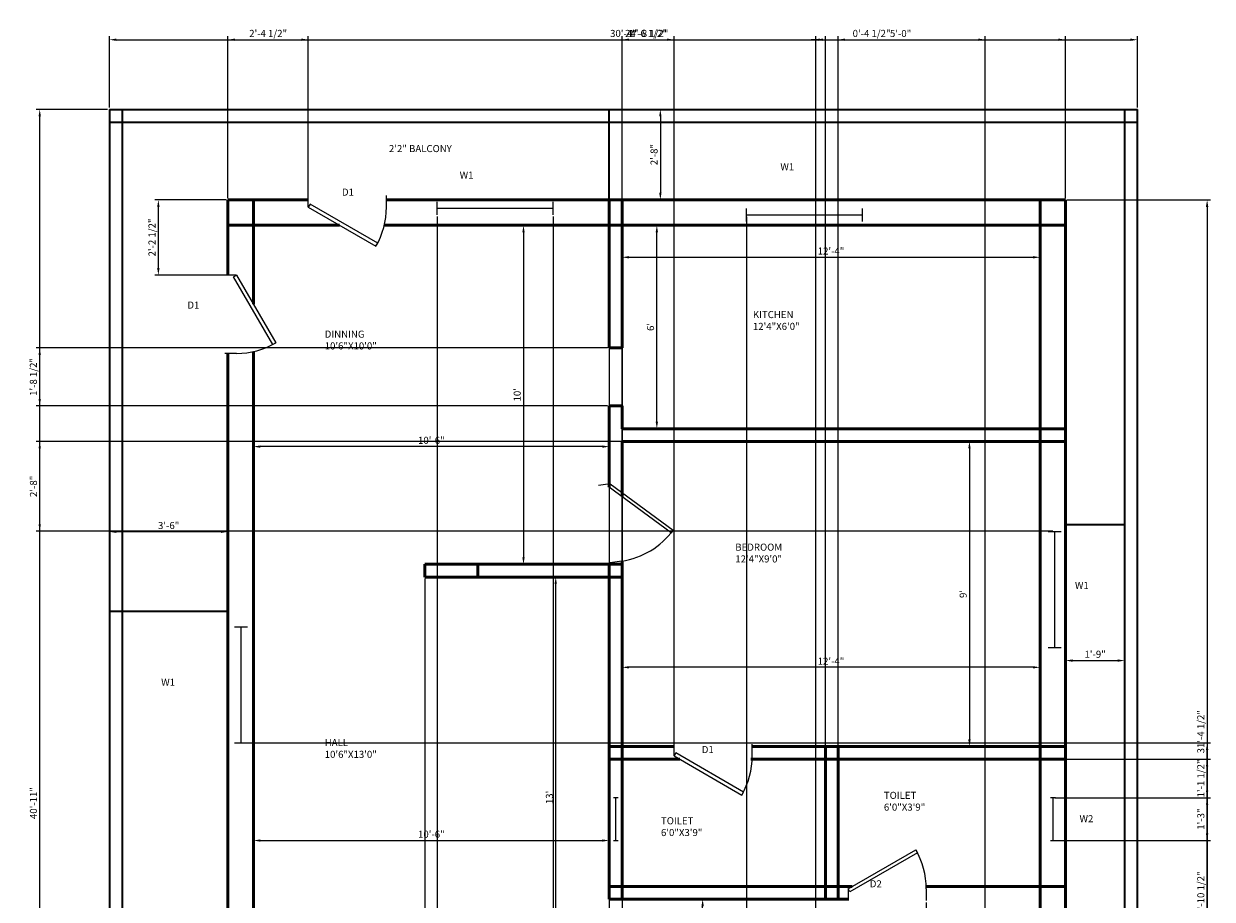
# Model space of a CAD drawing. Units: millimetres. Extents: x 2177 to 2598, y 1637 to 2185.
# Tile 2 of 2: x 2177 to 2598, y 1875 to 2185. Entities that reach past the tile are written whole.
import ezdxf

# ---------------------------------------------------------------- set-up
doc = ezdxf.new("R2010")
doc.units = ezdxf.units.MM
for name, color, linetype, lineweight in [('A-ANNO-DIMS', 150, 'Continuous', 18), ('A-ANNO-TEXT', 40, 'Continuous', 18), ('A-AREA-IDEN', 40, 'Continuous', 25), ('A-WALL-SITE', 100, 'Continuous', 35), ('door', 130, 'Continuous', 25), ('walls', 100, 'Continuous', 50), ('windows', 10, 'Continuous', 25)]:
    doc.layers.add(name, color=color, linetype=linetype, lineweight=lineweight)
doc.styles.get("Standard").update_dxf_attribs({"font": 'arial.ttf'})
doc.dimstyles.new('ISO-25', dxfattribs={"dimtxt": 2.5, "dimasz": 2.5, "dimexe": 1.25, "dimexo": 0.625, "dimtad": 1, "dimlunit": 3, "dimtxsty": 'Standard', "dimcen": 2.5, "dimadec": 0, "dimazin": 0, "dimtfac": 1, "dimtmove": 0, "dimatfit": 3, "dimfxl": 1, "dimarcsym": 0})

# ---------------------------------------------------------------- blocks, each defined once
blk = doc.blocks.new('*U2')
for p, q in [((0, 0), (0, -6)), ((40, 0), (40, -6))]:
    blk.add_line(p, q)
blk.add_lwpolyline([(0, 0), (34.64, 20), (35.52, 18.48), (0.87, -1.52)], close=True)
blk.add_arc((0, 0), 40, 0, 30)
blk = doc.blocks.new('*U4')
for p, q in [((0, 0), (0, -6)), ((40, 0), (40, -6))]:
    blk.add_line(p, q)
blk.add_lwpolyline([(0, 0), (28.28, 28.28), (29.52, 27.05), (1.24, -1.24)], close=True)
blk.add_arc((0, 0), 40, 0, 45)
blk = doc.blocks.new('*U3')
for p, q in [((0, 0), (0, 6)), ((40, 0), (40, 6))]:
    blk.add_line(p, q)
blk.add_lwpolyline([(0, 0), (34.64, -20), (35.52, -18.48), (0.87, 1.52)], close=True)
blk.add_arc((0, 0), 40, 330, 0)
blk = doc.blocks.new('*U7')
for p, q in [((0, 4), (0, 0)), ((36, 4), (36, 0)), ((0, 2), (36, 2))]:
    blk.add_line(p, q)
blk = doc.blocks.new('*D8')
at = {"layer": 'A-ANNO-DIMS', "color": 0, "lineweight": -2, "transparency": 16777216}
for p, q in [((2258.47, 2035.8), (2258.47, 2036.42)), ((2381.97, 2035.17), (2260.97, 2035.17)), ((2384.47, 2034.55), (2384.47, 2033.92))]:
    blk.add_line(p, q, dxfattribs=at)
at = {"layer": 'A-ANNO-DIMS', "color": 0, "transparency": 16777216}
for points in [[(2260.97, 2035.59), (2260.97, 2034.75), (2258.47, 2035.17)], [(2381.97, 2035.59), (2381.97, 2034.75), (2384.47, 2035.17)]]:
    blk.add_solid(points, dxfattribs=at)
at = {"layer": 'Defpoints', "color": 0, "transparency": 16777216}
for p in [(2258.47, 2035.17), (2258.47, 2035.17), (2384.47, 2035.17)]:
    blk.add_point(p, dxfattribs=at)
at = {"layer": 'A-ANNO-DIMS', "color": 0, "transparency": 16777216, "insert": (2321.47, 2037.07), "char_height": 2.5, "attachment_point": 5}
blk.add_mtext('10\'-6"', dxfattribs=at)
blk = doc.blocks.new('*D9')
at = {"layer": 'A-ANNO-DIMS', "color": 0, "lineweight": -2, "transparency": 16777216}
for p, q in [((2338.03, 2113.52), (2355.34, 2113.52)), ((2354.09, 2111.02), (2354.09, 1996.02)), ((2338.03, 1993.52), (2355.34, 1993.52))]:
    blk.add_line(p, q, dxfattribs=at)
at = {"layer": 'A-ANNO-DIMS', "color": 0, "transparency": 16777216}
for points in [[(2353.68, 2111.02), (2354.51, 2111.02), (2354.09, 2113.52)], [(2353.68, 1996.02), (2354.51, 1996.02), (2354.09, 1993.52)]]:
    blk.add_solid(points, dxfattribs=at)
at = {"layer": 'Defpoints', "color": 0, "transparency": 16777216}
for p in [(2337.4, 2113.52), (2337.4, 1993.52), (2354.09, 1993.52)]:
    blk.add_point(p, dxfattribs=at)
at = {"layer": 'A-ANNO-DIMS', "color": 0, "transparency": 16777216, "insert": (2352.19, 2053.52), "char_height": 2.5, "attachment_point": 5, "rotation": 90}
blk.add_mtext("10'", dxfattribs=at)
blk = doc.blocks.new('*D10')
at = {"layer": 'A-ANNO-DIMS', "color": 0, "lineweight": -2, "transparency": 16777216}
for p, q in [((2417.03, 2113.52), (2400.05, 2113.52)), ((2401.3, 2044.02), (2401.3, 2111.02)), ((2417.03, 2041.52), (2400.05, 2041.52))]:
    blk.add_line(p, q, dxfattribs=at)
at = {"layer": 'A-ANNO-DIMS', "color": 0, "transparency": 16777216}
for points in [[(2400.89, 2111.02), (2401.72, 2111.02), (2401.3, 2113.52)], [(2400.89, 2044.02), (2401.72, 2044.02), (2401.3, 2041.52)]]:
    blk.add_solid(points, dxfattribs=at)
at = {"layer": 'Defpoints', "color": 0, "transparency": 16777216}
for p in [(2401.3, 2113.52), (2417.66, 2113.52), (2417.66, 2041.52)]:
    blk.add_point(p, dxfattribs=at)
at = {"layer": 'A-ANNO-DIMS', "color": 0, "transparency": 16777216, "insert": (2399.4, 2077.52), "char_height": 2.5, "attachment_point": 5, "rotation": 90}
blk.add_mtext("6'", dxfattribs=at)
blk = doc.blocks.new('*D11')
at = {"layer": 'A-ANNO-DIMS', "color": 0, "lineweight": -2, "transparency": 16777216}
for p, q in [((2388.97, 2087.6), (2388.97, 2103.44)), ((2391.47, 2102.19), (2534.47, 2102.19)), ((2536.97, 2087.6), (2536.97, 2103.44))]:
    blk.add_line(p, q, dxfattribs=at)
at = {"layer": 'A-ANNO-DIMS', "color": 0, "transparency": 16777216}
for points in [[(2391.47, 2102.6), (2391.47, 2101.77), (2388.97, 2102.19)], [(2534.47, 2102.6), (2534.47, 2101.77), (2536.97, 2102.19)]]:
    blk.add_solid(points, dxfattribs=at)
at = {"layer": 'Defpoints', "color": 0, "transparency": 16777216}
for p in [(2536.97, 2102.19), (2388.97, 2086.97), (2536.97, 2086.97)]:
    blk.add_point(p, dxfattribs=at)
at = {"layer": 'A-ANNO-DIMS', "color": 0, "transparency": 16777216, "insert": (2462.97, 2104.07), "char_height": 2.5, "attachment_point": 5}
blk.add_mtext('12\'-4"', dxfattribs=at)
blk = doc.blocks.new('*D12')
at = {"layer": 'A-ANNO-DIMS', "color": 0, "lineweight": -2, "transparency": 16777216}
for p, q in [((2388.97, 1957.69), (2388.97, 1958.31)), ((2534.47, 1957.06), (2391.47, 1957.06)), ((2536.97, 1957.69), (2536.97, 1958.31))]:
    blk.add_line(p, q, dxfattribs=at)
at = {"layer": 'A-ANNO-DIMS', "color": 0, "transparency": 16777216}
for points in [[(2391.47, 1957.48), (2391.47, 1956.65), (2388.97, 1957.06)], [(2534.47, 1957.48), (2534.47, 1956.65), (2536.97, 1957.06)]]:
    blk.add_solid(points, dxfattribs=at)
at = {"layer": 'Defpoints', "color": 0, "transparency": 16777216}
for p in [(2388.97, 1957.06), (2388.97, 1957.06), (2536.97, 1957.06)]:
    blk.add_point(p, dxfattribs=at)
at = {"layer": 'A-ANNO-DIMS', "color": 0, "transparency": 16777216, "insert": (2462.97, 1958.94), "char_height": 2.5, "attachment_point": 5}
blk.add_mtext('12\'-4"', dxfattribs=at)
blk = doc.blocks.new('*D13')
at = {"layer": 'A-ANNO-DIMS', "color": 0, "lineweight": -2, "transparency": 16777216}
for p, q in [((2468.09, 2037.02), (2513.23, 2037.02)), ((2511.98, 2034.52), (2511.98, 1931.52)), ((2468.09, 1929.02), (2513.23, 1929.02))]:
    blk.add_line(p, q, dxfattribs=at)
at = {"layer": 'A-ANNO-DIMS', "color": 0, "transparency": 16777216}
for points in [[(2511.56, 2034.52), (2512.4, 2034.52), (2511.98, 2037.02)], [(2511.56, 1931.52), (2512.4, 1931.52), (2511.98, 1929.02)]]:
    blk.add_solid(points, dxfattribs=at)
at = {"layer": 'Defpoints', "color": 0, "transparency": 16777216}
for p in [(2467.47, 2037.02), (2467.47, 1929.02), (2511.98, 1929.02)]:
    blk.add_point(p, dxfattribs=at)
at = {"layer": 'A-ANNO-DIMS', "color": 0, "transparency": 16777216, "insert": (2510.08, 1983.02), "char_height": 2.5, "attachment_point": 5, "rotation": 90}
blk.add_mtext("9'", dxfattribs=at)
blk = doc.blocks.new('*D14')
at = {"layer": 'A-ANNO-DIMS', "color": 0, "lineweight": -2, "transparency": 16777216}
for p, q in [((2258.47, 1888.11), (2258.47, 1897.01)), ((2260.97, 1895.76), (2381.97, 1895.76)), ((2384.47, 1888.11), (2384.47, 1897.01))]:
    blk.add_line(p, q, dxfattribs=at)
at = {"layer": 'A-ANNO-DIMS', "color": 0, "transparency": 16777216}
for points in [[(2260.97, 1896.18), (2260.97, 1895.35), (2258.47, 1895.76)], [(2381.97, 1896.18), (2381.97, 1895.35), (2384.47, 1895.76)]]:
    blk.add_solid(points, dxfattribs=at)
at = {"layer": 'Defpoints', "color": 0, "transparency": 16777216}
for p in [(2384.47, 1895.76), (2258.47, 1887.49), (2384.47, 1887.49)]:
    blk.add_point(p, dxfattribs=at)
at = {"layer": 'A-ANNO-DIMS', "color": 0, "transparency": 16777216, "insert": (2321.47, 1897.67), "char_height": 2.5, "attachment_point": 5}
blk.add_mtext('10\'-6"', dxfattribs=at)
blk = doc.blocks.new('*D15')
at = {"layer": 'A-ANNO-DIMS', "color": 0, "lineweight": -2, "transparency": 16777216}
for p, q in [((2344.56, 1989.02), (2366.75, 1989.02)), ((2365.5, 1835.52), (2365.5, 1986.52)), ((2344.56, 1833.02), (2366.75, 1833.02))]:
    blk.add_line(p, q, dxfattribs=at)
at = {"layer": 'A-ANNO-DIMS', "color": 0, "transparency": 16777216}
for points in [[(2365.08, 1986.52), (2365.91, 1986.52), (2365.5, 1989.02)], [(2365.08, 1835.52), (2365.91, 1835.52), (2365.5, 1833.02)]]:
    blk.add_solid(points, dxfattribs=at)
at = {"layer": 'Defpoints', "color": 0, "transparency": 16777216}
for p in [(2343.93, 1989.02), (2365.5, 1989.02), (2343.93, 1833.02)]:
    blk.add_point(p, dxfattribs=at)
at = {"layer": 'A-ANNO-DIMS', "color": 0, "transparency": 16777216, "insert": (2363.59, 1911.02), "char_height": 2.5, "attachment_point": 5, "rotation": 90}
blk.add_mtext("13'", dxfattribs=at)
blk = doc.blocks.new('*D18')
at = {"layer": 'A-ANNO-DIMS', "color": 0, "lineweight": -2, "transparency": 16777216}
for p, q in [((2417.52, 1757.52), (2417.52, 1872.52)), ((2418.14, 1875.02), (2418.77, 1875.02)), ((2418.14, 1755.02), (2418.77, 1755.02))]:
    blk.add_line(p, q, dxfattribs=at)
at = {"layer": 'A-ANNO-DIMS', "color": 0, "transparency": 16777216}
for points in [[(2417.1, 1872.52), (2417.93, 1872.52), (2417.52, 1875.02)], [(2417.1, 1757.52), (2417.93, 1757.52), (2417.52, 1755.02)]]:
    blk.add_solid(points, dxfattribs=at)
at = {"layer": 'Defpoints', "color": 0, "transparency": 16777216}
for p in [(2417.52, 1875.02), (2417.52, 1875.02), (2417.52, 1755.02)]:
    blk.add_point(p, dxfattribs=at)
at = {"layer": 'A-ANNO-DIMS', "color": 0, "transparency": 16777216, "insert": (2415.61, 1815.02), "char_height": 2.5, "attachment_point": 5, "rotation": 90}
blk.add_mtext("10'", dxfattribs=at)
blk = doc.blocks.new('*D20')
at = {"layer": 'A-ANNO-DIMS', "color": 0, "lineweight": -2, "transparency": 16777216}
for p, q in [((2545.97, 1934.9), (2545.97, 1960.7)), ((2548.47, 1959.45), (2564.47, 1959.45)), ((2566.97, 1934.9), (2566.97, 1960.7))]:
    blk.add_line(p, q, dxfattribs=at)
at = {"layer": 'A-ANNO-DIMS', "color": 0, "transparency": 16777216}
for points in [[(2548.47, 1959.87), (2548.47, 1959.03), (2545.97, 1959.45)], [(2564.47, 1959.87), (2564.47, 1959.03), (2566.97, 1959.45)]]:
    blk.add_solid(points, dxfattribs=at)
at = {"layer": 'Defpoints', "color": 0, "transparency": 16777216}
for p in [(2566.97, 1959.45), (2545.97, 1934.27), (2566.97, 1934.27)]:
    blk.add_point(p, dxfattribs=at)
at = {"layer": 'A-ANNO-DIMS', "color": 0, "transparency": 16777216, "insert": (2556.47, 1961.35), "char_height": 2.5, "attachment_point": 5}
blk.add_mtext('1\'-9"', dxfattribs=at)
blk = doc.blocks.new('*D21')
at = {"layer": 'A-ANNO-DIMS', "color": 0, "lineweight": -2, "transparency": 16777216}
for p, q in [((2398.56, 2154.52), (2403.79, 2154.52)), ((2402.54, 2152.02), (2402.54, 2125.02)), ((2398.56, 2122.52), (2403.79, 2122.52))]:
    blk.add_line(p, q, dxfattribs=at)
at = {"layer": 'A-ANNO-DIMS', "color": 0, "transparency": 16777216}
for points in [[(2402.13, 2152.02), (2402.96, 2152.02), (2402.54, 2154.52)], [(2402.13, 2125.02), (2402.96, 2125.02), (2402.54, 2122.52)]]:
    blk.add_solid(points, dxfattribs=at)
at = {"layer": 'Defpoints', "color": 0, "transparency": 16777216}
for p in [(2397.93, 2154.52), (2397.93, 2122.52), (2402.54, 2122.52)]:
    blk.add_point(p, dxfattribs=at)
at = {"layer": 'A-ANNO-DIMS', "color": 0, "transparency": 16777216, "insert": (2400.64, 2138.52), "char_height": 2.5, "attachment_point": 5, "rotation": 90}
blk.add_mtext('2\'-8"', dxfattribs=at)
blk = doc.blocks.new('*D22')
at = {"layer": 'A-ANNO-DIMS', "color": 0, "lineweight": -2, "transparency": 16777216}
for p, q in [((2207.47, 1992.8), (2207.47, 2006.28)), ((2246.97, 2005.03), (2209.97, 2005.03)), ((2249.47, 1992.8), (2249.47, 2006.28))]:
    blk.add_line(p, q, dxfattribs=at)
at = {"layer": 'A-ANNO-DIMS', "color": 0, "transparency": 16777216}
for points in [[(2209.97, 2005.44), (2209.97, 2004.61), (2207.47, 2005.03)], [(2246.97, 2005.44), (2246.97, 2004.61), (2249.47, 2005.03)]]:
    blk.add_solid(points, dxfattribs=at)
at = {"layer": 'Defpoints', "color": 0, "transparency": 16777216}
for p in [(2207.47, 2005.03), (2207.47, 1992.17), (2249.47, 1992.17)]:
    blk.add_point(p, dxfattribs=at)
at = {"layer": 'A-ANNO-DIMS', "color": 0, "transparency": 16777216, "insert": (2228.47, 2006.93), "char_height": 2.5, "attachment_point": 5}
blk.add_mtext('3\'-6"', dxfattribs=at)
blk = doc.blocks.new('*D23')
at = {"layer": 'A-ANNO-DIMS', "color": 0, "lineweight": -2, "transparency": 16777216}
for p, q in [((2248.84, 2122.52), (2223.57, 2122.52)), ((2224.82, 2098.33), (2224.82, 2120.02)), ((2248.84, 2095.83), (2223.57, 2095.83))]:
    blk.add_line(p, q, dxfattribs=at)
at = {"layer": 'A-ANNO-DIMS', "color": 0, "transparency": 16777216}
for points in [[(2224.4, 2120.02), (2225.24, 2120.02), (2224.82, 2122.52)], [(2224.4, 2098.33), (2225.24, 2098.33), (2224.82, 2095.83)]]:
    blk.add_solid(points, dxfattribs=at)
at = {"layer": 'Defpoints', "color": 0, "transparency": 16777216}
for p in [(2224.82, 2122.52), (2249.47, 2122.52), (2249.47, 2095.83)]:
    blk.add_point(p, dxfattribs=at)
at = {"layer": 'A-ANNO-DIMS', "color": 0, "transparency": 16777216, "insert": (2222.9, 2109.18), "char_height": 2.5, "attachment_point": 5, "rotation": 90}
blk.add_mtext('2\'-2 1/2"', dxfattribs=at)
blk = doc.blocks.new('*D24')
at = {"layer": 'A-ANNO-DIMS', "color": 0, "lineweight": -2, "transparency": 16777216}
for p, q in [((2207.47, 2155.15), (2207.47, 2180.42)), ((2571.47, 2155.15), (2571.47, 2180.42)), ((2209.97, 2179.17), (2568.97, 2179.17))]:
    blk.add_line(p, q, dxfattribs=at)
at = {"layer": 'A-ANNO-DIMS', "color": 0, "transparency": 16777216}
for points in [[(2209.97, 2179.59), (2209.97, 2178.76), (2207.47, 2179.17)], [(2568.97, 2179.59), (2568.97, 2178.76), (2571.47, 2179.17)]]:
    blk.add_solid(points, dxfattribs=at)
at = {"layer": 'Defpoints', "color": 0, "transparency": 16777216}
for p in [(2571.47, 2179.17), (2207.47, 2154.52), (2571.47, 2154.52)]:
    blk.add_point(p, dxfattribs=at)
at = {"layer": 'A-ANNO-DIMS', "color": 0, "transparency": 16777216, "insert": (2389.47, 2181.08), "char_height": 2.5, "attachment_point": 5}
blk.add_mtext('30\'-4"', dxfattribs=at)
blk = doc.blocks.new('*D25')
at = {"layer": 'A-ANNO-DIMS', "color": 0, "lineweight": -2, "transparency": 16777216}
for p, q in [((2206.84, 2154.52), (2181.57, 2154.52)), ((2182.82, 1666.02), (2182.82, 2152.02)), ((2206.84, 1663.52), (2181.57, 1663.52))]:
    blk.add_line(p, q, dxfattribs=at)
at = {"layer": 'A-ANNO-DIMS', "color": 0, "transparency": 16777216}
for points in [[(2182.4, 2152.02), (2183.24, 2152.02), (2182.82, 2154.52)], [(2182.4, 1666.02), (2183.24, 1666.02), (2182.82, 1663.52)]]:
    blk.add_solid(points, dxfattribs=at)
at = {"layer": 'Defpoints', "color": 0, "transparency": 16777216}
for p in [(2182.82, 2154.52), (2207.47, 2154.52), (2207.47, 1663.52)]:
    blk.add_point(p, dxfattribs=at)
at = {"layer": 'A-ANNO-DIMS', "color": 0, "transparency": 16777216, "insert": (2180.92, 1909.02), "char_height": 2.5, "attachment_point": 5, "rotation": 90}
blk.add_mtext('40\'-11"', dxfattribs=at)
blk = doc.blocks.new('*D26')
at = {"layer": 'A-ANNO-DIMS', "color": 0, "lineweight": -2, "transparency": 16777216}
for p, q in [((2249.47, 2123.15), (2249.47, 2180.42)), ((2545.97, 2123.15), (2545.97, 2180.42)), ((2251.97, 2179.17), (2543.47, 2179.17))]:
    blk.add_line(p, q, dxfattribs=at)
at = {"layer": 'A-ANNO-DIMS', "color": 0, "transparency": 16777216}
for points in [[(2251.97, 2179.59), (2251.97, 2178.76), (2249.47, 2179.17)], [(2543.47, 2179.59), (2543.47, 2178.76), (2545.97, 2179.17)]]:
    blk.add_solid(points, dxfattribs=at)
at = {"layer": 'Defpoints', "color": 0, "transparency": 16777216}
for p in [(2545.97, 2179.17), (2249.47, 2122.52), (2545.97, 2122.52)]:
    blk.add_point(p, dxfattribs=at)
at = {"layer": 'A-ANNO-DIMS', "color": 0, "transparency": 16777216, "insert": (2397.72, 2181.09), "char_height": 2.5, "attachment_point": 5}
blk.add_mtext('24\'-8 1/2"', dxfattribs=at)
blk = doc.blocks.new('*D27')
at = {"layer": 'A-ANNO-DIMS', "color": 0, "lineweight": -2, "transparency": 16777216}
for p, q in [((2546.59, 2122.52), (2597.37, 2122.52)), ((2596.12, 2120.02), (2596.12, 1748.52)), ((2546.59, 1746.02), (2597.37, 1746.02))]:
    blk.add_line(p, q, dxfattribs=at)
at = {"layer": 'A-ANNO-DIMS', "color": 0, "transparency": 16777216}
for points in [[(2595.7, 2120.02), (2596.54, 2120.02), (2596.12, 2122.52)], [(2595.7, 1748.52), (2596.54, 1748.52), (2596.12, 1746.02)]]:
    blk.add_solid(points, dxfattribs=at)
at = {"layer": 'Defpoints', "color": 0, "transparency": 16777216}
for p in [(2545.97, 2122.52), (2545.97, 1746.02), (2596.12, 1746.02)]:
    blk.add_point(p, dxfattribs=at)
at = {"layer": 'A-ANNO-DIMS', "color": 0, "transparency": 16777216, "insert": (2594.2, 1934.27), "char_height": 2.5, "attachment_point": 5, "rotation": 90}
blk.add_mtext('31\'-4 1/2"', dxfattribs=at)
blk = doc.blocks.new('*D29')
at = {"layer": 'A-ANNO-DIMS', "color": 0, "lineweight": -2, "transparency": 16777216}
for p, q in [((2460.97, 1929.65), (2460.97, 2180.42)), ((2465.47, 1929.65), (2465.47, 2180.42)), ((2458.47, 2179.17), (2455.97, 2179.17)), ((2460.97, 2179.17), (2465.47, 2179.17)), ((2467.97, 2179.17), (2484.19, 2179.17))]:
    blk.add_line(p, q, dxfattribs=at)
at = {"layer": 'A-ANNO-DIMS', "color": 0, "transparency": 16777216}
for points in [[(2458.47, 2179.59), (2458.47, 2178.76), (2460.97, 2179.17)], [(2467.97, 2179.59), (2467.97, 2178.76), (2465.47, 2179.17)]]:
    blk.add_solid(points, dxfattribs=at)
at = {"layer": 'Defpoints', "color": 0, "transparency": 16777216}
for p in [(2465.47, 2179.17), (2460.97, 1929.02), (2465.47, 1929.02)]:
    blk.add_point(p, dxfattribs=at)
at = {"layer": 'A-ANNO-DIMS', "color": 0, "transparency": 16777216, "insert": (2477.33, 2181.09), "char_height": 2.5, "attachment_point": 5}
blk.add_mtext('0\'-4 1/2"', dxfattribs=at)
blk = doc.blocks.new('*D33')
at = {"layer": 'A-ANNO-DIMS', "color": 0, "lineweight": -2, "transparency": 16777216}
for p, q in [((2323.55, 2116.57), (2323.55, 1637.62)), ((2364.65, 2116.57), (2364.65, 1637.62)), ((2326.05, 1638.87), (2362.15, 1638.87))]:
    blk.add_line(p, q, dxfattribs=at)
at = {"layer": 'A-ANNO-DIMS', "color": 0, "transparency": 16777216}
for points in [[(2326.05, 1639.29), (2326.05, 1638.46), (2323.55, 1638.87)], [(2362.15, 1639.29), (2362.15, 1638.46), (2364.65, 1638.87)]]:
    blk.add_solid(points, dxfattribs=at)
at = {"layer": 'Defpoints', "color": 0, "transparency": 16777216}
for p in [(2323.55, 2117.19), (2364.65, 2117.19), (2364.65, 1638.87)]:
    blk.add_point(p, dxfattribs=at)
at = {"layer": 'A-ANNO-DIMS', "color": 0, "transparency": 16777216, "insert": (2344.1, 1640.78), "char_height": 2.5, "attachment_point": 5}
blk.add_mtext('3\'-5"', dxfattribs=at)
blk = doc.blocks.new('*D34')
at = {"layer": 'A-ANNO-DIMS', "color": 0, "lineweight": -2, "transparency": 16777216}
for p, q in [((2542.2, 1910.93), (2597.37, 1910.93)), ((2596.12, 1908.43), (2596.12, 1898.25)), ((2542.2, 1895.75), (2597.37, 1895.75))]:
    blk.add_line(p, q, dxfattribs=at)
at = {"layer": 'A-ANNO-DIMS', "color": 0, "transparency": 16777216}
for points in [[(2595.7, 1908.43), (2596.54, 1908.43), (2596.12, 1910.93)], [(2595.7, 1898.25), (2596.54, 1898.25), (2596.12, 1895.75)]]:
    blk.add_solid(points, dxfattribs=at)
at = {"layer": 'Defpoints', "color": 0, "transparency": 16777216}
for p in [(2541.57, 1910.93), (2541.57, 1895.75), (2596.12, 1895.75)]:
    blk.add_point(p, dxfattribs=at)
at = {"layer": 'A-ANNO-DIMS', "color": 0, "transparency": 16777216, "insert": (2594.22, 1903.34), "char_height": 2.5, "attachment_point": 5, "rotation": 90}
blk.add_mtext('1\'-3"', dxfattribs=at)
blk = doc.blocks.new('*D35')
at = {"layer": 'A-ANNO-DIMS', "color": 0, "lineweight": -2, "transparency": 16777216}
for p, q in [((2457.6, 1746.65), (2457.6, 2180.42)), ((2517.6, 1746.65), (2517.6, 2180.42)), ((2460.1, 2179.17), (2515.1, 2179.17))]:
    blk.add_line(p, q, dxfattribs=at)
at = {"layer": 'A-ANNO-DIMS', "color": 0, "transparency": 16777216}
for points in [[(2460.1, 2179.59), (2460.1, 2178.76), (2457.6, 2179.17)], [(2515.1, 2179.59), (2515.1, 2178.76), (2517.6, 2179.17)]]:
    blk.add_solid(points, dxfattribs=at)
at = {"layer": 'Defpoints', "color": 0, "transparency": 16777216}
for p in [(2517.6, 2179.17), (2457.6, 1746.02), (2517.6, 1746.02)]:
    blk.add_point(p, dxfattribs=at)
at = {"layer": 'A-ANNO-DIMS', "color": 0, "transparency": 16777216, "insert": (2487.6, 2181.07), "char_height": 2.5, "attachment_point": 5}
blk.add_mtext('5\'-0"', dxfattribs=at)
blk = doc.blocks.new('*D42')
at = {"layer": 'A-ANNO-DIMS', "color": 0, "lineweight": -2, "transparency": 16777216}
for p, q in [((2388.97, 1929.65), (2388.97, 2180.42)), ((2407.39, 1929.65), (2407.39, 2180.42)), ((2391.47, 2179.17), (2404.89, 2179.17))]:
    blk.add_line(p, q, dxfattribs=at)
at = {"layer": 'A-ANNO-DIMS', "color": 0, "transparency": 16777216}
for points in [[(2391.47, 2179.59), (2391.47, 2178.76), (2388.97, 2179.17)], [(2404.89, 2179.59), (2404.89, 2178.76), (2407.39, 2179.17)]]:
    blk.add_solid(points, dxfattribs=at)
at = {"layer": 'Defpoints', "color": 0, "transparency": 16777216}
for p in [(2407.39, 2179.17), (2388.97, 1929.02), (2407.39, 1929.02)]:
    blk.add_point(p, dxfattribs=at)
at = {"layer": 'A-ANNO-DIMS', "color": 0, "transparency": 16777216, "insert": (2398.18, 2181.09), "char_height": 2.5, "attachment_point": 5}
blk.add_mtext('1\'-6 1/2"', dxfattribs=at)
blk = doc.blocks.new('*D43')
at = {"layer": 'A-ANNO-DIMS', "color": 0, "lineweight": -2, "transparency": 16777216}
for p, q in [((2545.97, 1878.9), (2545.97, 1637.62)), ((2496.67, 1873.88), (2496.67, 1637.62)), ((2499.17, 1638.87), (2543.47, 1638.87))]:
    blk.add_line(p, q, dxfattribs=at)
at = {"layer": 'A-ANNO-DIMS', "color": 0, "transparency": 16777216}
for points in [[(2499.17, 1639.29), (2499.17, 1638.46), (2496.67, 1638.87)], [(2543.47, 1639.29), (2543.47, 1638.46), (2545.97, 1638.87)]]:
    blk.add_solid(points, dxfattribs=at)
at = {"layer": 'Defpoints', "color": 0, "transparency": 16777216}
for p in [(2545.97, 1879.52), (2496.67, 1874.51), (2545.97, 1638.87)]:
    blk.add_point(p, dxfattribs=at)
at = {"layer": 'A-ANNO-DIMS', "color": 0, "transparency": 16777216, "insert": (2521.32, 1640.79), "char_height": 2.5, "attachment_point": 5}
blk.add_mtext('4\'-1 1/2"', dxfattribs=at)
blk = doc.blocks.new('*D44')
at = {"layer": 'A-ANNO-DIMS', "color": 0, "lineweight": -2, "transparency": 16777216}
for p, q in [((2546.59, 1924.52), (2597.37, 1924.52)), ((2596.12, 1913.43), (2596.12, 1922.02)), ((2542.2, 1910.93), (2597.37, 1910.93))]:
    blk.add_line(p, q, dxfattribs=at)
at = {"layer": 'A-ANNO-DIMS', "color": 0, "transparency": 16777216}
for points in [[(2595.7, 1922.02), (2596.54, 1922.02), (2596.12, 1924.52)], [(2595.7, 1913.43), (2596.54, 1913.43), (2596.12, 1910.93)]]:
    blk.add_solid(points, dxfattribs=at)
at = {"layer": 'Defpoints', "color": 0, "transparency": 16777216}
for p in [(2545.97, 1924.52), (2596.12, 1924.52), (2541.57, 1910.93)]:
    blk.add_point(p, dxfattribs=at)
at = {"layer": 'A-ANNO-DIMS', "color": 0, "transparency": 16777216, "insert": (2594.2, 1917.73), "char_height": 2.5, "attachment_point": 5, "rotation": 90}
blk.add_mtext('1\'-1 1/2"', dxfattribs=at)
blk = doc.blocks.new('*D46')
at = {"layer": 'A-ANNO-DIMS', "color": 0, "lineweight": -2, "transparency": 16777216}
for p, q in [((2383.84, 2070.11), (2181.57, 2070.11)), ((2182.82, 2052.05), (2182.82, 2067.61)), ((2383.84, 2049.55), (2181.57, 2049.55))]:
    blk.add_line(p, q, dxfattribs=at)
at = {"layer": 'A-ANNO-DIMS', "color": 0, "transparency": 16777216}
for points in [[(2182.4, 2067.61), (2183.24, 2067.61), (2182.82, 2070.11)], [(2182.4, 2052.05), (2183.24, 2052.05), (2182.82, 2049.55)]]:
    blk.add_solid(points, dxfattribs=at)
at = {"layer": 'Defpoints', "color": 0, "transparency": 16777216}
for p in [(2182.82, 2070.11), (2384.47, 2070.11), (2384.47, 2049.55)]:
    blk.add_point(p, dxfattribs=at)
at = {"layer": 'A-ANNO-DIMS', "color": 0, "transparency": 16777216, "insert": (2180.9, 2059.83), "char_height": 2.5, "attachment_point": 5, "rotation": 90}
blk.add_mtext('1\'-8 1/2"', dxfattribs=at)
blk = doc.blocks.new('*D47')
at = {"layer": 'A-ANNO-DIMS', "color": 0, "lineweight": -2, "transparency": 16777216}
for p, q in [((2319.22, 1988.4), (2319.22, 1637.62)), ((2388.97, 1988.4), (2388.97, 1637.62)), ((2321.72, 1638.87), (2386.47, 1638.87))]:
    blk.add_line(p, q, dxfattribs=at)
at = {"layer": 'A-ANNO-DIMS', "color": 0, "transparency": 16777216}
for points in [[(2321.72, 1639.29), (2321.72, 1638.46), (2319.22, 1638.87)], [(2386.47, 1639.29), (2386.47, 1638.46), (2388.97, 1638.87)]]:
    blk.add_solid(points, dxfattribs=at)
at = {"layer": 'Defpoints', "color": 0, "transparency": 16777216}
for p in [(2319.22, 1989.02), (2388.97, 1989.02), (2388.97, 1638.87)]:
    blk.add_point(p, dxfattribs=at)
at = {"layer": 'A-ANNO-DIMS', "color": 0, "transparency": 16777216, "insert": (2354.09, 1640.77), "char_height": 2.5, "attachment_point": 5}
blk.add_mtext('5\'-10"', dxfattribs=at)
blk = doc.blocks.new('*D48')
at = {"layer": 'A-ANNO-DIMS', "color": 0, "lineweight": -2, "transparency": 16777216}
for p, q in [((2388.97, 2121.9), (2388.97, 1637.62)), ((2433.07, 2116.49), (2433.07, 1637.62)), ((2391.47, 1638.87), (2430.57, 1638.87))]:
    blk.add_line(p, q, dxfattribs=at)
at = {"layer": 'A-ANNO-DIMS', "color": 0, "transparency": 16777216}
for points in [[(2391.47, 1639.29), (2391.47, 1638.46), (2388.97, 1638.87)], [(2430.57, 1639.29), (2430.57, 1638.46), (2433.07, 1638.87)]]:
    blk.add_solid(points, dxfattribs=at)
at = {"layer": 'Defpoints', "color": 0, "transparency": 16777216}
for p in [(2388.97, 2122.52), (2433.07, 2117.11), (2433.07, 1638.87)]:
    blk.add_point(p, dxfattribs=at)
at = {"layer": 'A-ANNO-DIMS', "color": 0, "transparency": 16777216, "insert": (2411.02, 1640.78), "char_height": 2.5, "attachment_point": 5}
blk.add_mtext('3\'-8"', dxfattribs=at)
blk = doc.blocks.new('*D49')
at = {"layer": 'A-ANNO-DIMS', "color": 0, "lineweight": -2, "transparency": 16777216}
for p, q in [((2249.47, 2123.15), (2249.47, 2180.42)), ((2277.91, 2123.15), (2277.91, 2180.42)), ((2251.97, 2179.17), (2275.41, 2179.17))]:
    blk.add_line(p, q, dxfattribs=at)
at = {"layer": 'A-ANNO-DIMS', "color": 0, "transparency": 16777216}
for points in [[(2251.97, 2179.59), (2251.97, 2178.76), (2249.47, 2179.17)], [(2275.41, 2179.59), (2275.41, 2178.76), (2277.91, 2179.17)]]:
    blk.add_solid(points, dxfattribs=at)
at = {"layer": 'Defpoints', "color": 0, "transparency": 16777216}
for p in [(2277.91, 2179.17), (2249.47, 2122.52), (2277.91, 2122.52)]:
    blk.add_point(p, dxfattribs=at)
at = {"layer": 'A-ANNO-DIMS', "color": 0, "transparency": 16777216, "insert": (2263.69, 2181.09), "char_height": 2.5, "attachment_point": 5}
blk.add_mtext('2\'-4 1/2"', dxfattribs=at)
blk = doc.blocks.new('*D50')
at = {"layer": 'A-ANNO-DIMS', "color": 0, "lineweight": -2, "transparency": 16777216}
for p, q in [((2254.73, 1930.31), (2597.37, 1930.31)), ((2596.12, 1826.52), (2596.12, 1927.81)), ((2259.09, 1824.02), (2597.37, 1824.02))]:
    blk.add_line(p, q, dxfattribs=at)
at = {"layer": 'A-ANNO-DIMS', "color": 0, "transparency": 16777216}
for points in [[(2595.7, 1927.81), (2596.54, 1927.81), (2596.12, 1930.31)], [(2595.7, 1826.52), (2596.54, 1826.52), (2596.12, 1824.02)]]:
    blk.add_solid(points, dxfattribs=at)
at = {"layer": 'Defpoints', "color": 0, "transparency": 16777216}
for p in [(2254.11, 1930.31), (2596.12, 1930.31), (2258.47, 1824.02)]:
    blk.add_point(p, dxfattribs=at)
at = {"layer": 'A-ANNO-DIMS', "color": 0, "transparency": 16777216, "insert": (2594.2, 1877.17), "char_height": 2.5, "attachment_point": 5, "rotation": 90}
blk.add_mtext('8\'-10 1/2"', dxfattribs=at)
blk = doc.blocks.new('*D51')
at = {"layer": 'A-ANNO-DIMS', "color": 0, "lineweight": -2, "transparency": 16777216}
for p, q in [((2545.34, 2037.02), (2181.57, 2037.02)), ((2182.82, 2007.69), (2182.82, 2034.52)), ((2541.54, 2005.19), (2181.57, 2005.19))]:
    blk.add_line(p, q, dxfattribs=at)
at = {"layer": 'A-ANNO-DIMS', "color": 0, "transparency": 16777216}
for points in [[(2182.4, 2034.52), (2183.24, 2034.52), (2182.82, 2037.02)], [(2182.4, 2007.69), (2183.24, 2007.69), (2182.82, 2005.19)]]:
    blk.add_solid(points, dxfattribs=at)
at = {"layer": 'Defpoints', "color": 0, "transparency": 16777216}
for p in [(2182.82, 2037.02), (2545.97, 2037.02), (2542.17, 2005.19)]:
    blk.add_point(p, dxfattribs=at)
at = {"layer": 'A-ANNO-DIMS', "color": 0, "transparency": 16777216, "insert": (2180.92, 2021.11), "char_height": 2.5, "attachment_point": 5, "rotation": 90}
blk.add_mtext('2\'-8"', dxfattribs=at)
blk = doc.blocks.new('*D53')
at = {"layer": 'A-ANNO-DIMS', "color": 0, "lineweight": -2, "transparency": 16777216}
for p, q in [((2384.47, 2121.9), (2384.47, 1637.62)), ((2364.65, 2116.57), (2364.65, 1637.62)), ((2367.15, 1638.87), (2381.97, 1638.87))]:
    blk.add_line(p, q, dxfattribs=at)
at = {"layer": 'A-ANNO-DIMS', "color": 0, "transparency": 16777216}
for points in [[(2367.15, 1639.29), (2367.15, 1638.46), (2364.65, 1638.87)], [(2381.97, 1639.29), (2381.97, 1638.46), (2384.47, 1638.87)]]:
    blk.add_solid(points, dxfattribs=at)
at = {"layer": 'Defpoints', "color": 0, "transparency": 16777216}
for p in [(2384.47, 2122.52), (2364.65, 2117.19), (2384.47, 1638.87)]:
    blk.add_point(p, dxfattribs=at)
at = {"layer": 'A-ANNO-DIMS', "color": 0, "transparency": 16777216, "insert": (2374.56, 1640.77), "char_height": 2.5, "attachment_point": 5}
blk.add_mtext('1\'-8"', dxfattribs=at)

msp = doc.modelspace()

# ---------------------------------------------------------------- linework, layer by layer
at = {"layer": 'A-WALL-SITE'}
for p, q in [((2207.47, 2154.523), (2207.47, 1663.523)), ((2207.47, 2154.523), (2571.47, 2154.523)), ((2211.97, 2154.523), (2211.97, 1668.023)), ((2384.47, 2122.523), (2384.47, 2154.523)), ((2566.97, 1663.523), (2566.97, 2154.523)), ((2571.47, 1663.523), (2571.47, 2154.523)), ((2207.47, 2150.023), (2571.47, 2150.023)), ((2545.97, 2007.63), (2566.97, 2007.63)), ((2249.47, 1976.834), (2207.47, 1976.834))]:
    msp.add_line(p, q, dxfattribs=at)
at = {"layer": 'walls'}
for p, q in [((2249.47, 2122.523), (2249.47, 2095.834)), ((2249.47, 2122.523), (2277.908, 2122.523)), ((2258.47, 2122.523), (2258.47, 2085.551)), ((2305.574, 2122.523), (2545.97, 2122.523)), ((2384.47, 2122.523), (2384.47, 2070.113)), ((2388.97, 2122.523), (2388.97, 2070.113)), ((2536.97, 2122.523), (2536.97, 1746.023)), ((2545.97, 2122.523), (2545.97, 1746.023)), ((2249.47, 2113.523), (2288.98, 2113.523)), ((2304.826, 2113.523), (2545.97, 2113.523)), ((2249.47, 2068.167), (2249.47, 1824.023)), ((2258.47, 2068.811), (2258.47, 1824.023)), ((2384.47, 2070.113), (2388.97, 2070.113)), ((2384.47, 2049.555), (2388.97, 2049.555)), ((2384.47, 2049.555), (2384.47, 2020.786)), ((2388.97, 2049.555), (2388.97, 2041.523)), ((2388.97, 2041.523), (2545.97, 2041.523)), ((2388.97, 2037.023), (2545.97, 2037.023)), ((2388.97, 2037.023), (2388.97, 2017.46)), ((2388.97, 1994.686), (2388.97, 1875.023)), ((2319.22, 1993.523), (2319.22, 1989.023)), ((2319.22, 1993.523), (2388.97, 1993.523)), ((2337.97, 1993.523), (2337.97, 1989.023)), ((2384.47, 1993.523), (2384.47, 1875.023)), ((2319.22, 1989.023), (2388.97, 1989.023)), ((2384.47, 1929.023), (2388.97, 1929.023)), ((2388.97, 1929.023), (2407.388, 1929.023)), ((2435.055, 1929.023), (2545.97, 1929.023)), ((2460.97, 1929.023), (2460.97, 1875.023)), ((2465.47, 1929.023), (2465.47, 1875.023)), ((2384.47, 1924.523), (2409.428, 1924.523)), ((2434.543, 1924.523), (2545.97, 1924.523)), ((2384.47, 1879.523), (2470.508, 1879.523)), ((2496.759, 1879.523), (2545.97, 1879.523)), ((2384.47, 1875.023), (2469.006, 1875.023))]:
    msp.add_line(p, q, dxfattribs=at)

# ---------------------------------------------------------------- block references
at = {"layer": 'door', "xscale": 0.6916711511996688, "yscale": 0.6916711511996688, "zscale": 0.6916711511996688}
for name, p in [('*U3', (2277.908, 2119.916)), ('*U3', (2407.388, 1925.695)), ('*U2', (2469.006, 1878.656))]:
    msp.add_blockref(name, p, dxfattribs=at)
at = {"layer": 'door'}
for name, p, xscale, yscale, zscale, rotation in [('*U2', (2252.533, 2095.834), 0.6916711511996688, 0.6916711511996688, 0.6916711511996688, 270), ('*U4', (2384.811, 2022.039), 0.6916711511996687, 0.6916711511996687, 0.6916711511996687, 278.5282782366667)]:
    msp.add_blockref(name, p, dxfattribs=dict(at, xscale=xscale, yscale=yscale, zscale=zscale, rotation=rotation))
at = {"layer": 'windows'}
for p, xscale, yscale, zscale, rotation in [((2364.645, 2121.759), 1.141567510768898, 1.141567510768898, 1.141567510768898, 180), ((2474.168, 2119.397), 1.141567510768898, 1.141567510768898, 1.141567510768898, 180), ((2544.448, 1964.091), 1.141567510768898, 1.141567510768898, 1.141567510768898, 90), ((2256.391, 1930.313), 1.141567510768898, 1.141567510768898, 1.141567510768898, 90), ((2387.602, 1895.752), 0.4216643708746738, 0.4216643708746738, 0.4216643708746738, 90), ((2542.415, 1895.752), 0.4216643708746738, 0.4216643708746738, 0.4216643708746738, 90)]:
    msp.add_blockref('*U7', p, dxfattribs=dict(at, xscale=xscale, yscale=yscale, zscale=zscale, rotation=rotation))

# ---------------------------------------------------------------- texts
at = {"layer": 'A-ANNO-TEXT', "char_height": 2.5, "attachment_point": 1}
for s, width, insert in [('W1', 19.70711, (2445.037, 2135.463)), ('W1', 18.82473, (2331.5, 2132.524)), ('D1', 15.75188, (2289.823, 2126.49)), ('D1', 8.63437, (2235.11, 2086.516)), ('W1', 8.22484, (2549.335, 1987.313)), ('W1', 15.25017, (2225.83, 1953.011)), ('D1', 10.8018, (2417.215, 1929.2)), ('W2', 16.01962, (2550.95, 1904.741)), ('D2', 19.97339, (2476.7, 1881.701))]:
    msp.add_mtext_dynamic_manual_height_columns(s, width=width, gutter_width=12.5, heights=[0], dxfattribs=dict(at, insert=insert))
at = {"layer": 'A-AREA-IDEN', "char_height": 2.5, "attachment_point": 1}
for s, width, insert in [('2\'2" BALCONY', 62.76176, (2306.46, 2141.901)), ('KITCHEN\\P12\'4"X6\'0"', 47.75853, (2435.304, 2083.144)), ('DINNING\\P10\'6"X10\'0"', 70.59948, (2283.723, 2076.228)), ('BEDROOM\\P12\'4"X9\'0"', 74.06023, (2429.074, 2000.839)), ('HALL\\P10\'6"X13\'0"', 74.75239, (2283.723, 1931.675)), ('TOILET\\P6\'0"X3\'9"', 35.29974, (2481.678, 1913.001)), ('TOILET\\P6\'0"X3\'9"', 39.45265, (2402.773, 1904.01))]:
    msp.add_mtext_dynamic_manual_height_columns(s, width=width, gutter_width=12.5, heights=[0], dxfattribs=dict(at, insert=insert))

# ---------------------------------------------------------------- dimensions: what is measured, and where the dimension line sits
at = {"layer": 'A-ANNO-DIMS'}
for base, p1, p2, override, picture, middle in [((2545.97, 2179.173), (2249.47, 2122.523), (2545.97, 2122.523), {"dimdec": 1, "dimlfac": 1, "dimrnd": 0, "dimzin": 1, "dimdsep": 46, "dimlunit": 4, "dimfrac": 2}, '*D26', (2397.72, 2181.091)), ((2277.908, 2179.173), (2249.47, 2122.523), (2277.908, 2122.523), {"dimdec": 1, "dimlfac": 1, "dimrnd": 0, "dimzin": 1, "dimdsep": 46, "dimlunit": 4, "dimfrac": 2}, '*D49', (2263.689, 2181.091)), ((2407.388, 2179.173), (2388.97, 1929.023), (2407.388, 1929.023), {"dimdec": 1, "dimlfac": 1, "dimrnd": 0, "dimzin": 1, "dimdsep": 46, "dimlunit": 4, "dimfrac": 2}, '*D42', (2398.179, 2181.091)), ((2465.47, 2179.173), (2460.97, 1929.023), (2465.47, 1929.023), {"dimdec": 1, "dimlfac": 1, "dimrnd": 0, "dimzin": 1, "dimdsep": 46, "dimlunit": 4, "dimfrac": 2}, '*D29', (2477.33, 2181.091)), ((2571.47, 2179.173), (2207.47, 2154.523), (2571.47, 2154.523), {"dimdec": 1, "dimlfac": 1, "dimrnd": 0, "dimzin": 1, "dimdsep": 46, "dimlunit": 4, "dimfrac": 2}, '*D24', (2389.47, 2181.075)), ((2517.598, 2179.173), (2457.598, 1746.023), (2517.598, 1746.023), {"dimdec": 1, "dimlfac": 1, "dimrnd": 0, "dimzin": 1, "dimdsep": 46, "dimlunit": 4, "dimfrac": 2}, '*D35', (2487.598, 2181.074)), ((2384.47, 1638.873), (2364.645, 2117.193), (2384.47, 2122.523), {"dimdec": 1, "dimlfac": 1, "dimrnd": 0, "dimzin": 1, "dimdsep": 46, "dimlunit": 4, "dimfrac": 2}, '*D53', (2374.558, 1640.774)), ((2433.071, 1638.873), (2388.97, 2122.523), (2433.071, 2117.114), {"dimdec": 1, "dimlfac": 1, "dimrnd": 0, "dimzin": 1, "dimdsep": 46, "dimlunit": 4, "dimfrac": 2}, '*D48', (2411.02, 1640.775)), ((2364.645, 1638.873), (2323.549, 2117.193), (2364.645, 2117.193), {"dimdec": 1, "dimlfac": 1, "dimrnd": 0, "dimzin": 1, "dimdsep": 46, "dimlunit": 4, "dimfrac": 2}, '*D33', (2344.097, 1640.775)), ((2536.97, 2102.185), (2388.97, 2086.971), (2536.97, 2086.971), {"dimclrd": 0, "dimclre": 0, "dimclrt": 0}, '*D11', (2462.97, 2104.065)), ((2258.47, 2035.17), (2384.47, 2035.17), (2258.47, 2035.17), {"dimclrd": 0, "dimclre": 0, "dimclrt": 0}, '*D8', (2321.47, 2037.072)), ((2207.47, 2005.027), (2249.47, 1992.171), (2207.47, 1992.171), {"dimclrd": 0, "dimclre": 0, "dimclrt": 0}, '*D22', (2228.47, 2006.93)), ((2388.969775, 1638.87304), (2319.219775, 1989.02304), (2388.969775, 1989.02304), {"dimdec": 1, "dimlfac": 1, "dimrnd": 0, "dimzin": 1, "dimdsep": 46, "dimlunit": 4, "dimfrac": 2}, '*D47', (2354.094775, 1640.774472469)), ((2566.97, 1959.449), (2545.97, 1934.273), (2566.97, 1934.273), {"dimclrd": 0, "dimclre": 0, "dimclrt": 0}, '*D20', (2556.47, 1961.351)), ((2388.97, 1957.065), (2536.97, 1957.065), (2388.97, 1957.065), {"dimclrd": 0, "dimclre": 0, "dimclrt": 0}, '*D12', (2462.97, 1958.945)), ((2384.47, 1895.764), (2258.47, 1887.486), (2384.47, 1887.486), {"dimclrd": 0, "dimclre": 0, "dimclrt": 0}, '*D14', (2321.47, 1897.665)), ((2545.97, 1638.873), (2496.673, 1874.506), (2545.97, 1879.523), {"dimdec": 1, "dimlfac": 1, "dimrnd": 0, "dimzin": 1, "dimdsep": 46, "dimlunit": 4, "dimfrac": 2}, '*D43', (2521.322, 1640.791))]:
    dim = msp.add_linear_dim(base=base, p1=p1, p2=p2, dimstyle='ISO-25', override=override, dxfattribs=at)
    dim.commit()
    dim.dimension.update_dxf_attribs({"geometry": picture, "text_midpoint": middle})
for base, p1, p2, override, picture, middle in [((2182.82, 2154.523), (2207.47, 1663.523), (2207.47, 2154.523), {"dimdec": 1, "dimlfac": 1, "dimrnd": 0, "dimzin": 1, "dimdsep": 46, "dimlunit": 4, "dimfrac": 2}, '*D25', (2180.918, 1909.023)), ((2402.545, 2122.523), (2397.93, 2154.523), (2397.93, 2122.523), {"dimclrd": 0, "dimclre": 0, "dimclrt": 0}, '*D21', (2400.643, 2138.523)), ((2224.82, 2122.523), (2249.47, 2095.834), (2249.47, 2122.523), {"dimdec": 1, "dimlfac": 1, "dimrnd": 0, "dimzin": 1, "dimdsep": 46, "dimlunit": 4, "dimfrac": 2}, '*D23', (2222.902, 2109.178)), ((2596.12, 1746.023), (2545.97, 2122.523), (2545.97, 1746.023), {"dimdec": 1, "dimlfac": 1, "dimrnd": 0, "dimzin": 1, "dimdsep": 46, "dimlunit": 4, "dimfrac": 2}, '*D27', (2594.201, 1934.273)), ((2354.095, 1993.523), (2337.403, 2113.523), (2337.403, 1993.523), {"dimclrd": 0, "dimclre": 0, "dimclrt": 0}, '*D9', (2352.193, 2053.523)), ((2401.302, 2113.523), (2417.655, 2041.523), (2417.655, 2113.523), {"dimclrd": 0, "dimclre": 0, "dimclrt": 0}, '*D10', (2399.401, 2077.523)), ((2182.82, 2070.113), (2384.47, 2049.555), (2384.47, 2070.113), {"dimdec": 1, "dimlfac": 1, "dimrnd": 0, "dimzin": 1, "dimdsep": 46, "dimlunit": 4, "dimfrac": 2}, '*D46', (2180.902, 2059.834)), ((2182.82, 2037.023), (2542.165, 2005.187), (2545.97, 2037.023), {"dimdec": 1, "dimlfac": 1, "dimrnd": 0, "dimzin": 1, "dimdsep": 46, "dimlunit": 4, "dimfrac": 2}, '*D51', (2180.918, 2021.105)), ((2511.98, 1929.023), (2467.47, 2037.023), (2467.47, 1929.023), {"dimclrd": 0, "dimclre": 0, "dimclrt": 0}, '*D13', (2510.079, 1983.023)), ((2365.495, 1989.023), (2343.933, 1833.023), (2343.933, 1989.023), {"dimclrd": 0, "dimclre": 0, "dimclrt": 0}, '*D15', (2363.593, 1911.023)), ((2596.12, 1930.313), (2258.47, 1824.023), (2254.108, 1930.313), {"dimdec": 1, "dimlfac": 1, "dimrnd": 0, "dimzin": 1, "dimdsep": 46, "dimlunit": 4, "dimfrac": 2}, '*D50', (2594.202, 1877.168)), ((2596.12, 1924.523), (2541.572, 1910.932), (2545.97, 1924.523), {"dimdec": 1, "dimlfac": 1, "dimrnd": 0, "dimzin": 1, "dimdsep": 46, "dimlunit": 4, "dimfrac": 2}, '*D44', (2594.202, 1917.728)), ((2596.12, 1895.752), (2541.572, 1910.932), (2541.572, 1895.752), {"dimdec": 1, "dimlfac": 1, "dimrnd": 0, "dimzin": 1, "dimdsep": 46, "dimlunit": 4, "dimfrac": 2}, '*D34', (2594.217, 1903.342)), ((2417.515, 1875.023), (2417.515, 1755.023), (2417.515, 1875.023), {"dimclrd": 0, "dimclre": 0, "dimclrt": 0}, '*D18', (2415.614, 1815.023))]:
    dim = msp.add_linear_dim(base=base, p1=p1, p2=p2, angle=90, dimstyle='ISO-25', override=override, dxfattribs=at)
    dim.commit()
    dim.dimension.update_dxf_attribs({"geometry": picture, "text_midpoint": middle})

doc.saveas('drawing.dxf')
